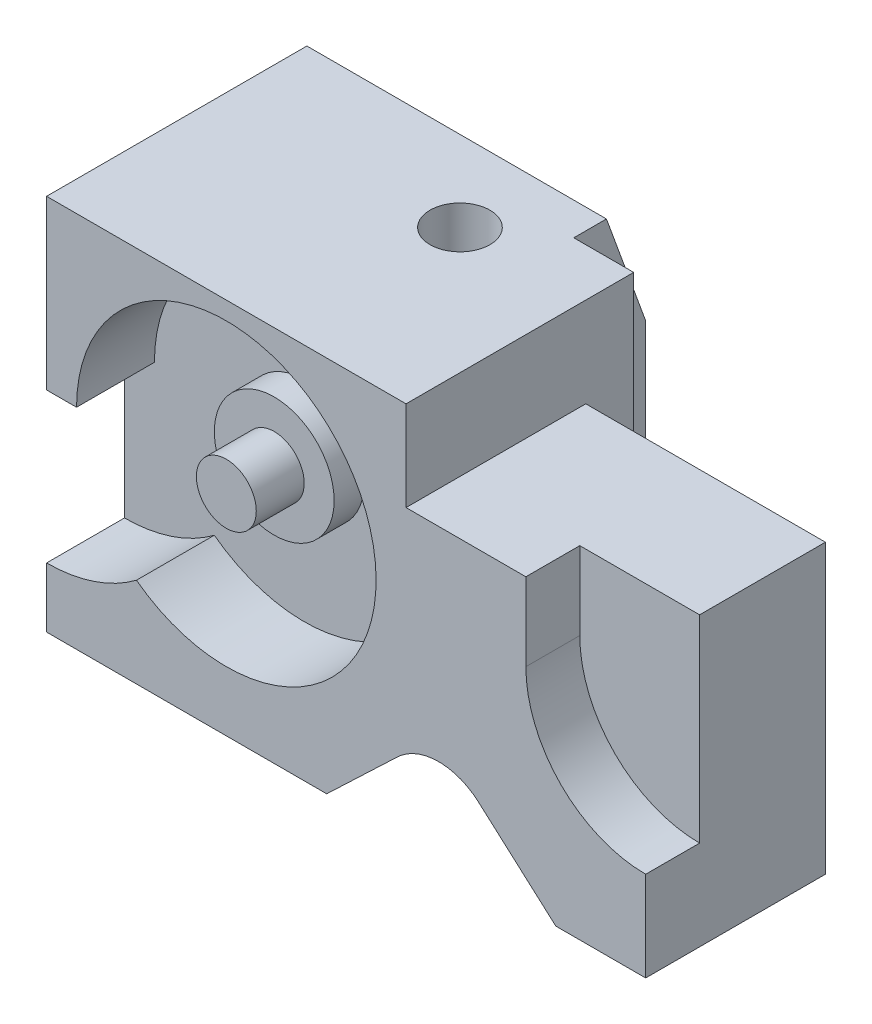
ISO-10303-21;
HEADER;
FILE_DESCRIPTION(('STEP AP214'),'2;1');
FILE_NAME('part.step','',(''),(''),'','','');
FILE_SCHEMA(('AUTOMOTIVE_DESIGN { 1 0 10303 214 1 1 1 1 }'));
ENDSEC;
DATA;
#1=APPLICATION_CONTEXT('core data for automotive mechanical design processes');
#2=APPLICATION_PROTOCOL_DEFINITION('international standard','automotive_design',2000,#1);
#3=PRODUCT_CONTEXT('',#1,'mechanical');
#4=PRODUCT('Part','Part','',(#3));
#5=PRODUCT_RELATED_PRODUCT_CATEGORY('part','',(#4));
#6=PRODUCT_DEFINITION_FORMATION('','',#4);
#7=PRODUCT_DEFINITION_CONTEXT('part definition',#1,'design');
#8=PRODUCT_DEFINITION('design','',#6,#7);
#9=PRODUCT_DEFINITION_SHAPE('','',#8);
#10=(LENGTH_UNIT() NAMED_UNIT(*) SI_UNIT(.MILLI.,.METRE.));
#11=(NAMED_UNIT(*) PLANE_ANGLE_UNIT() SI_UNIT($,.RADIAN.));
#12=(NAMED_UNIT(*) SI_UNIT($,.STERADIAN.) SOLID_ANGLE_UNIT());
#13=UNCERTAINTY_MEASURE_WITH_UNIT(LENGTH_MEASURE(1.E-05),#10,'distance_accuracy_value','');
#14=(GEOMETRIC_REPRESENTATION_CONTEXT(3) GLOBAL_UNCERTAINTY_ASSIGNED_CONTEXT((#13)) GLOBAL_UNIT_ASSIGNED_CONTEXT((#10,
#11,#12)) REPRESENTATION_CONTEXT('',''));
#15=CARTESIAN_POINT('',(0.,0.,0.));
#16=DIRECTION('',(0.,0.,1.));
#17=DIRECTION('',(1.,0.,0.));
#18=AXIS2_PLACEMENT_3D('',#15,#16,#17);
#19=CARTESIAN_POINT('',(-50.,63.,25.));
#20=DIRECTION('',(0.,0.,-1.));
#21=DIRECTION('',(-1.,0.,0.));
#22=AXIS2_PLACEMENT_3D('',#19,#20,#21);
#23=PLANE('',#22);
#24=DIRECTION('',(1.,0.,0.));
#25=VECTOR('',#24,1.);
#26=CARTESIAN_POINT('',(0.,35.,25.));
#27=LINE('',#26,#25);
#28=CARTESIAN_POINT('',(-50.,35.,25.));
#29=VERTEX_POINT('',#28);
#30=CARTESIAN_POINT('',(-45.,35.,25.));
#31=VERTEX_POINT('',#30);
#32=EDGE_CURVE('E266',#29,#31,#27,.T.);
#33=ORIENTED_EDGE('',*,*,#32,.T.);
#34=CARTESIAN_POINT('',(-20.,35.,25.));
#35=DIRECTION('',(0.,0.,1.));
#36=DIRECTION('',(1.,0.,0.));
#37=AXIS2_PLACEMENT_3D('',#34,#35,#36);
#38=CIRCLE('',#37,25.);
#39=CARTESIAN_POINT('',(-35.,15.,25.));
#40=VERTEX_POINT('',#39);
#41=EDGE_CURVE('E292',#40,#31,#38,.T.);
#42=ORIENTED_EDGE('',*,*,#41,.F.);
#43=CARTESIAN_POINT('',(-50.,35.,25.));
#44=DIRECTION('',(0.,0.,1.));
#45=DIRECTION('',(1.,0.,0.));
#46=AXIS2_PLACEMENT_3D('',#43,#44,#45);
#47=CIRCLE('',#46,25.);
#48=CARTESIAN_POINT('',(-50.,10.,25.));
#49=VERTEX_POINT('',#48);
#50=EDGE_CURVE('E264',#49,#40,#47,.T.);
#51=ORIENTED_EDGE('',*,*,#50,.F.);
#52=DIRECTION('',(0.,-1.,0.));
#53=VECTOR('',#52,1.);
#54=CARTESIAN_POINT('',(-50.,63.,25.));
#55=LINE('',#54,#53);
#56=CARTESIAN_POINT('',(-50.,0.,25.));
#57=VERTEX_POINT('',#56);
#58=EDGE_CURVE('E209',#49,#57,#55,.T.);
#59=ORIENTED_EDGE('',*,*,#58,.T.);
#60=DIRECTION('',(1.,0.,0.));
#61=VECTOR('',#60,1.);
#62=CARTESIAN_POINT('',(-50.,0.,25.));
#63=LINE('',#62,#61);
#64=CARTESIAN_POINT('',(-3.24667991345898,0.,25.));
#65=VERTEX_POINT('',#64);
#66=EDGE_CURVE('E351',#57,#65,#63,.T.);
#67=ORIENTED_EDGE('',*,*,#66,.T.);
#68=DIRECTION('',(0.724485251032931,0.689290302438494,0.));
#69=VECTOR('',#68,1.);
#70=CARTESIAN_POINT('',(-1.54256620012688,1.62132915083853,25.));
#71=LINE('',#70,#69);
#72=CARTESIAN_POINT('',(8.34365992738258,11.0272898487142,25.));
#73=VERTEX_POINT('',#72);
#74=EDGE_CURVE('E336',#65,#73,#71,.T.);
#75=ORIENTED_EDGE('',*,*,#74,.T.);
#76=CARTESIAN_POINT('',(15.4582363295416,4.,25.));
#77=DIRECTION('',(0.,0.,1.));
#78=DIRECTION('',(1.,0.,0.));
#79=AXIS2_PLACEMENT_3D('',#76,#77,#78);
#80=CIRCLE('',#79,9.99999999999999);
#81=CARTESIAN_POINT('',(22.1048169338786,11.4714768466516,25.));
#82=VERTEX_POINT('',#81);
#83=EDGE_CURVE('E335',#82,#73,#80,.T.);
#84=ORIENTED_EDGE('',*,*,#83,.F.);
#85=DIRECTION('',(0.747147684665161,-0.664658060433701,0.));
#86=VECTOR('',#85,1.);
#87=CARTESIAN_POINT('',(15.4619618054821,17.3809205831477,25.));
#88=LINE('',#87,#86);
#89=CARTESIAN_POINT('',(35.,0.,25.));
#90=VERTEX_POINT('',#89);
#91=EDGE_CURVE('E331',#82,#90,#88,.T.);
#92=ORIENTED_EDGE('',*,*,#91,.T.);
#93=CARTESIAN_POINT('',(50.,0.,25.));
#94=VERTEX_POINT('',#93);
#95=EDGE_CURVE('E359',#90,#94,#63,.T.);
#96=ORIENTED_EDGE('',*,*,#95,.T.);
#97=DIRECTION('',(0.,-1.,0.));
#98=VECTOR('',#97,1.);
#99=CARTESIAN_POINT('',(50.,63.,25.));
#100=LINE('',#99,#98);
#101=CARTESIAN_POINT('',(50.,15.,25.));
#102=VERTEX_POINT('',#101);
#103=EDGE_CURVE('E353',#102,#94,#100,.T.);
#104=ORIENTED_EDGE('',*,*,#103,.F.);
#105=CARTESIAN_POINT('',(50.,35.,25.));
#106=DIRECTION('',(0.,0.,1.));
#107=DIRECTION('',(1.,0.,0.));
#108=AXIS2_PLACEMENT_3D('',#105,#106,#107);
#109=CIRCLE('',#108,20.);
#110=CARTESIAN_POINT('',(30.,35.,25.));
#111=VERTEX_POINT('',#110);
#112=EDGE_CURVE('E319',#111,#102,#109,.T.);
#113=ORIENTED_EDGE('',*,*,#112,.F.);
#114=DIRECTION('',(0.,1.,0.));
#115=VECTOR('',#114,1.);
#116=CARTESIAN_POINT('',(30.,0.,25.));
#117=LINE('',#116,#115);
#118=CARTESIAN_POINT('',(30.,48.,25.));
#119=VERTEX_POINT('',#118);
#120=EDGE_CURVE('E312',#111,#119,#117,.T.);
#121=ORIENTED_EDGE('',*,*,#120,.T.);
#122=DIRECTION('',(1.,0.,0.));
#123=VECTOR('',#122,1.);
#124=CARTESIAN_POINT('',(50.,48.,25.));
#125=LINE('',#124,#123);
#126=CARTESIAN_POINT('',(10.,48.,25.));
#127=VERTEX_POINT('',#126);
#128=EDGE_CURVE('E304',#127,#119,#125,.T.);
#129=ORIENTED_EDGE('',*,*,#128,.F.);
#130=DIRECTION('',(0.,1.,0.));
#131=VECTOR('',#130,1.);
#132=CARTESIAN_POINT('',(10.,48.,25.));
#133=LINE('',#132,#131);
#134=CARTESIAN_POINT('',(10.,63.,25.));
#135=VERTEX_POINT('',#134);
#136=EDGE_CURVE('E310',#127,#135,#133,.T.);
#137=ORIENTED_EDGE('',*,*,#136,.T.);
#138=DIRECTION('',(1.,0.,0.));
#139=VECTOR('',#138,1.);
#140=CARTESIAN_POINT('',(-50.,63.,25.));
#141=LINE('',#140,#139);
#142=CARTESIAN_POINT('',(-50.,63.,25.));
#143=VERTEX_POINT('',#142);
#144=EDGE_CURVE('E348',#143,#135,#141,.T.);
#145=ORIENTED_EDGE('',*,*,#144,.F.);
#146=EDGE_CURVE('E203',#143,#29,#55,.T.);
#147=ORIENTED_EDGE('',*,*,#146,.T.);
#148=EDGE_LOOP('',(#33,#42,#51,#59,#67,#75,#84,#92,#96,#104,#113,#121,#129,#137,#145,#147));
#149=FACE_BOUND('',#148,.T.);
#150=ADVANCED_FACE('F39',(#149),#23,.F.);
#151=CARTESIAN_POINT('',(-50.,63.,-25.));
#152=DIRECTION('',(1.,0.,0.));
#153=DIRECTION('',(0.,0.,-1.));
#154=AXIS2_PLACEMENT_3D('',#151,#152,#153);
#155=PLANE('',#154);
#156=DIRECTION('',(0.,0.,1.));
#157=VECTOR('',#156,1.);
#158=CARTESIAN_POINT('',(-50.,63.,-25.));
#159=LINE('',#158,#157);
#160=CARTESIAN_POINT('',(-50.,63.,-18.4485357832084));
#161=VERTEX_POINT('',#160);
#162=EDGE_CURVE('E197',#161,#143,#159,.T.);
#163=ORIENTED_EDGE('',*,*,#162,.F.);
#164=DIRECTION('',(0.,0.93969262078591,0.342020143325666));
#165=VECTOR('',#164,1.);
#166=CARTESIAN_POINT('',(-50.,45.,-25.));
#167=LINE('',#166,#165);
#168=CARTESIAN_POINT('',(-50.,45.,-25.));
#169=VERTEX_POINT('',#168);
#170=EDGE_CURVE('E182',#169,#161,#167,.T.);
#171=ORIENTED_EDGE('',*,*,#170,.F.);
#172=DIRECTION('',(0.,-1.,0.));
#173=VECTOR('',#172,1.);
#174=CARTESIAN_POINT('',(-50.,63.,-25.));
#175=LINE('',#174,#173);
#176=CARTESIAN_POINT('',(-50.,0.,-25.));
#177=VERTEX_POINT('',#176);
#178=EDGE_CURVE('E195',#169,#177,#175,.T.);
#179=ORIENTED_EDGE('',*,*,#178,.T.);
#180=DIRECTION('',(0.,0.,1.));
#181=VECTOR('',#180,1.);
#182=CARTESIAN_POINT('',(-50.,0.,-25.));
#183=LINE('',#182,#181);
#184=EDGE_CURVE('E356',#177,#57,#183,.T.);
#185=ORIENTED_EDGE('',*,*,#184,.T.);
#186=ORIENTED_EDGE('',*,*,#58,.F.);
#187=DIRECTION('',(0.,0.,1.));
#188=VECTOR('',#187,1.);
#189=CARTESIAN_POINT('',(-50.,10.,12.));
#190=LINE('',#189,#188);
#191=CARTESIAN_POINT('',(-50.,10.,12.));
#192=VERTEX_POINT('',#191);
#193=EDGE_CURVE('E270',#192,#49,#190,.T.);
#194=ORIENTED_EDGE('',*,*,#193,.F.);
#195=DIRECTION('',(0.,-1.,0.));
#196=VECTOR('',#195,1.);
#197=CARTESIAN_POINT('',(-50.,0.,12.));
#198=LINE('',#197,#196);
#199=CARTESIAN_POINT('',(-50.,35.,12.));
#200=VERTEX_POINT('',#199);
#201=EDGE_CURVE('E261',#200,#192,#198,.T.);
#202=ORIENTED_EDGE('',*,*,#201,.F.);
#203=DIRECTION('',(0.,0.,1.));
#204=VECTOR('',#203,1.);
#205=CARTESIAN_POINT('',(-50.,35.,12.));
#206=LINE('',#205,#204);
#207=EDGE_CURVE('E274',#200,#29,#206,.T.);
#208=ORIENTED_EDGE('',*,*,#207,.T.);
#209=ORIENTED_EDGE('',*,*,#146,.F.);
#210=EDGE_LOOP('',(#163,#171,#179,#185,#186,#194,#202,#208,#209));
#211=FACE_BOUND('',#210,.T.);
#212=ADVANCED_FACE('F194',(#211),#155,.F.);
#213=CARTESIAN_POINT('',(-20.,35.,12.));
#214=DIRECTION('',(0.,0.,1.));
#215=DIRECTION('',(1.,0.,0.));
#216=AXIS2_PLACEMENT_3D('',#213,#214,#215);
#217=CYLINDRICAL_SURFACE('',#216,25.);
#218=DIRECTION('',(0.,0.,1.));
#219=VECTOR('',#218,1.);
#220=CARTESIAN_POINT('',(-45.,35.,12.));
#221=LINE('',#220,#219);
#222=CARTESIAN_POINT('',(-45.,35.,12.));
#223=VERTEX_POINT('',#222);
#224=EDGE_CURVE('E280',#223,#31,#221,.T.);
#225=ORIENTED_EDGE('',*,*,#224,.F.);
#226=CARTESIAN_POINT('',(-20.,35.,12.));
#227=DIRECTION('',(0.,0.,1.));
#228=DIRECTION('',(1.,0.,0.));
#229=AXIS2_PLACEMENT_3D('',#226,#227,#228);
#230=CIRCLE('',#229,25.);
#231=CARTESIAN_POINT('',(-35.,15.,12.));
#232=VERTEX_POINT('',#231);
#233=EDGE_CURVE('E294',#232,#223,#230,.T.);
#234=ORIENTED_EDGE('',*,*,#233,.F.);
#235=DIRECTION('',(0.,0.,1.));
#236=VECTOR('',#235,1.);
#237=CARTESIAN_POINT('',(-35.,15.,12.));
#238=LINE('',#237,#236);
#239=EDGE_CURVE('E277',#232,#40,#238,.T.);
#240=ORIENTED_EDGE('',*,*,#239,.T.);
#241=ORIENTED_EDGE('',*,*,#41,.T.);
#242=EDGE_LOOP('',(#225,#234,#240,#241));
#243=FACE_BOUND('',#242,.T.);
#244=ADVANCED_FACE('F432',(#243),#217,.F.);
#245=CARTESIAN_POINT('',(0.,63.,0.));
#246=DIRECTION('',(0.,1.,0.));
#247=DIRECTION('',(0.,0.,1.));
#248=AXIS2_PLACEMENT_3D('',#245,#246,#247);
#249=PLANE('',#248);
#250=DIRECTION('',(-1.,0.,0.));
#251=VECTOR('',#250,1.);
#252=CARTESIAN_POINT('',(67.,63.,-18.4485357832084));
#253=LINE('',#252,#251);
#254=CARTESIAN_POINT('',(0.,63.,-18.4485357832084));
#255=VERTEX_POINT('',#254);
#256=EDGE_CURVE('E53',#255,#161,#253,.T.);
#257=ORIENTED_EDGE('',*,*,#256,.T.);
#258=ORIENTED_EDGE('',*,*,#162,.T.);
#259=ORIENTED_EDGE('',*,*,#144,.T.);
#260=DIRECTION('',(0.,0.,1.));
#261=VECTOR('',#260,1.);
#262=CARTESIAN_POINT('',(10.,63.,25.));
#263=LINE('',#262,#261);
#264=CARTESIAN_POINT('',(10.,63.,-13.));
#265=VERTEX_POINT('',#264);
#266=EDGE_CURVE('E300',#265,#135,#263,.T.);
#267=ORIENTED_EDGE('',*,*,#266,.F.);
#268=DIRECTION('',(1.,0.,0.));
#269=VECTOR('',#268,1.);
#270=CARTESIAN_POINT('',(10.,63.,-13.));
#271=LINE('',#270,#269);
#272=CARTESIAN_POINT('',(0.,63.,-13.));
#273=VERTEX_POINT('',#272);
#274=EDGE_CURVE('E247',#273,#265,#271,.T.);
#275=ORIENTED_EDGE('',*,*,#274,.F.);
#276=DIRECTION('',(0.,0.,1.));
#277=VECTOR('',#276,1.);
#278=CARTESIAN_POINT('',(0.,63.,-13.));
#279=LINE('',#278,#277);
#280=EDGE_CURVE('E246',#255,#273,#279,.T.);
#281=ORIENTED_EDGE('',*,*,#280,.F.);
#282=EDGE_LOOP('',(#257,#258,#259,#267,#275,#281));
#283=FACE_BOUND('',#282,.T.);
#284=CARTESIAN_POINT('',(-11.,63.,-4.99999999999998));
#285=DIRECTION('',(0.,1.,0.));
#286=DIRECTION('',(0.,0.,1.));
#287=AXIS2_PLACEMENT_3D('',#284,#285,#286);
#288=CIRCLE('',#287,5.);
#289=CARTESIAN_POINT('',(-11.,63.,0.));
#290=VERTEX_POINT('',#289);
#291=EDGE_CURVE('E218',#290,#290,#288,.T.);
#292=ORIENTED_EDGE('',*,*,#291,.F.);
#293=EDGE_LOOP('',(#292));
#294=FACE_BOUND('',#293,.T.);
#295=ADVANCED_FACE('F425',(#283,#294),#249,.T.);
#296=CARTESIAN_POINT('',(50.,63.,-25.));
#297=DIRECTION('',(0.,0.,1.));
#298=DIRECTION('',(1.,0.,0.));
#299=AXIS2_PLACEMENT_3D('',#296,#297,#298);
#300=PLANE('',#299);
#301=ORIENTED_EDGE('',*,*,#178,.F.);
#302=DIRECTION('',(-1.,0.,0.));
#303=VECTOR('',#302,1.);
#304=CARTESIAN_POINT('',(67.,45.,-25.));
#305=LINE('',#304,#303);
#306=CARTESIAN_POINT('',(0.,45.,-25.));
#307=VERTEX_POINT('',#306);
#308=EDGE_CURVE('E179',#307,#169,#305,.T.);
#309=ORIENTED_EDGE('',*,*,#308,.F.);
#310=DIRECTION('',(0.,1.,0.));
#311=VECTOR('',#310,1.);
#312=CARTESIAN_POINT('',(0.,-54.,-25.));
#313=LINE('',#312,#311);
#314=CARTESIAN_POINT('',(0.,3.08895864516005,-25.));
#315=VERTEX_POINT('',#314);
#316=EDGE_CURVE('E252',#315,#307,#313,.T.);
#317=ORIENTED_EDGE('',*,*,#316,.F.);
#318=DIRECTION('',(0.724485251032931,0.689290302438494,0.));
#319=VECTOR('',#318,1.);
#320=CARTESIAN_POINT('',(56.1623591892788,56.5229926659267,-25.));
#321=LINE('',#320,#319);
#322=CARTESIAN_POINT('',(-3.24667991345898,0.,-25.));
#323=VERTEX_POINT('',#322);
#324=EDGE_CURVE('E343',#323,#315,#321,.T.);
#325=ORIENTED_EDGE('',*,*,#324,.F.);
#326=DIRECTION('',(-1.,0.,0.));
#327=VECTOR('',#326,1.);
#328=CARTESIAN_POINT('',(50.,0.,-25.));
#329=LINE('',#328,#327);
#330=EDGE_CURVE('E201',#323,#177,#329,.T.);
#331=ORIENTED_EDGE('',*,*,#330,.T.);
#332=EDGE_LOOP('',(#301,#309,#317,#325,#331));
#333=FACE_BOUND('',#332,.T.);
#334=ADVANCED_FACE('F199',(#333),#300,.F.);
#335=CARTESIAN_POINT('',(0.,0.,0.));
#336=DIRECTION('',(0.,1.,0.));
#337=DIRECTION('',(0.,0.,1.));
#338=AXIS2_PLACEMENT_3D('',#335,#336,#337);
#339=PLANE('',#338);
#340=DIRECTION('',(0.,0.,1.));
#341=VECTOR('',#340,1.);
#342=CARTESIAN_POINT('',(35.,0.,0.));
#343=LINE('',#342,#341);
#344=CARTESIAN_POINT('',(35.,0.,-4.99999999999998));
#345=VERTEX_POINT('',#344);
#346=EDGE_CURVE('E207',#345,#90,#343,.T.);
#347=ORIENTED_EDGE('',*,*,#346,.F.);
#348=DIRECTION('',(1.,0.,0.));
#349=VECTOR('',#348,1.);
#350=CARTESIAN_POINT('',(0.,0.,-4.99999999999998));
#351=LINE('',#350,#349);
#352=CARTESIAN_POINT('',(50.,0.,-4.99999999999998));
#353=VERTEX_POINT('',#352);
#354=EDGE_CURVE('E243',#345,#353,#351,.T.);
#355=ORIENTED_EDGE('',*,*,#354,.T.);
#356=DIRECTION('',(0.,0.,-1.));
#357=VECTOR('',#356,1.);
#358=CARTESIAN_POINT('',(50.,0.,0.));
#359=LINE('',#358,#357);
#360=EDGE_CURVE('E349',#94,#353,#359,.T.);
#361=ORIENTED_EDGE('',*,*,#360,.F.);
#362=ORIENTED_EDGE('',*,*,#95,.F.);
#363=EDGE_LOOP('',(#347,#355,#361,#362));
#364=FACE_BOUND('',#363,.T.);
#365=ADVANCED_FACE('F391',(#364),#339,.F.);
#366=CARTESIAN_POINT('',(-11.,0.,-4.99999999999998));
#367=DIRECTION('',(0.,1.,0.));
#368=DIRECTION('',(0.,0.,1.));
#369=AXIS2_PLACEMENT_3D('',#366,#367,#368);
#370=CIRCLE('',#369,5.);
#371=CARTESIAN_POINT('',(-11.,0.,0.));
#372=VERTEX_POINT('',#371);
#373=EDGE_CURVE('E220',#372,#372,#370,.T.);
#374=ORIENTED_EDGE('',*,*,#373,.T.);
#375=EDGE_LOOP('',(#374));
#376=FACE_BOUND('',#375,.T.);
#377=DIRECTION('',(0.,0.,-1.));
#378=VECTOR('',#377,1.);
#379=CARTESIAN_POINT('',(-3.24667991345897,0.,0.));
#380=LINE('',#379,#378);
#381=EDGE_CURVE('E204',#65,#323,#380,.T.);
#382=ORIENTED_EDGE('',*,*,#381,.F.);
#383=ORIENTED_EDGE('',*,*,#66,.F.);
#384=ORIENTED_EDGE('',*,*,#184,.F.);
#385=ORIENTED_EDGE('',*,*,#330,.F.);
#386=EDGE_LOOP('',(#382,#383,#384,#385));
#387=FACE_BOUND('',#386,.T.);
#388=ADVANCED_FACE('F373',(#376,#387),#339,.F.);
#389=CARTESIAN_POINT('',(50.,63.,0.));
#390=DIRECTION('',(-1.,0.,0.));
#391=DIRECTION('',(0.,0.,1.));
#392=AXIS2_PLACEMENT_3D('',#389,#390,#391);
#393=PLANE('',#392);
#394=ORIENTED_EDGE('',*,*,#360,.T.);
#395=DIRECTION('',(0.,1.,0.));
#396=VECTOR('',#395,1.);
#397=CARTESIAN_POINT('',(50.,-69.,-4.99999999999998));
#398=LINE('',#397,#396);
#399=CARTESIAN_POINT('',(50.,48.,-4.99999999999998));
#400=VERTEX_POINT('',#399);
#401=EDGE_CURVE('E224',#353,#400,#398,.T.);
#402=ORIENTED_EDGE('',*,*,#401,.T.);
#403=DIRECTION('',(0.,0.,-1.));
#404=VECTOR('',#403,1.);
#405=CARTESIAN_POINT('',(50.,48.,-25.));
#406=LINE('',#405,#404);
#407=CARTESIAN_POINT('',(50.,48.,16.));
#408=VERTEX_POINT('',#407);
#409=EDGE_CURVE('E297',#408,#400,#406,.T.);
#410=ORIENTED_EDGE('',*,*,#409,.F.);
#411=DIRECTION('',(0.,1.,0.));
#412=VECTOR('',#411,1.);
#413=CARTESIAN_POINT('',(50.,0.,16.));
#414=LINE('',#413,#412);
#415=CARTESIAN_POINT('',(50.,15.,16.));
#416=VERTEX_POINT('',#415);
#417=EDGE_CURVE('E324',#416,#408,#414,.T.);
#418=ORIENTED_EDGE('',*,*,#417,.F.);
#419=DIRECTION('',(0.,0.,1.));
#420=VECTOR('',#419,1.);
#421=CARTESIAN_POINT('',(50.,15.,16.));
#422=LINE('',#421,#420);
#423=EDGE_CURVE('E329',#416,#102,#422,.T.);
#424=ORIENTED_EDGE('',*,*,#423,.T.);
#425=ORIENTED_EDGE('',*,*,#103,.T.);
#426=EDGE_LOOP('',(#394,#402,#410,#418,#424,#425));
#427=FACE_BOUND('',#426,.T.);
#428=ADVANCED_FACE('F41',(#427),#393,.F.);
#429=CARTESIAN_POINT('',(15.4582363295416,4.,-38.));
#430=DIRECTION('',(0.,0.,1.));
#431=DIRECTION('',(1.,0.,0.));
#432=AXIS2_PLACEMENT_3D('',#429,#430,#431);
#433=CYLINDRICAL_SURFACE('',#432,9.99999999999999);
#434=CARTESIAN_POINT('',(15.4582363295416,4.,-13.));
#435=DIRECTION('',(0.,0.,1.));
#436=DIRECTION('',(1.,0.,0.));
#437=AXIS2_PLACEMENT_3D('',#434,#435,#436);
#438=CIRCLE('',#437,9.99999999999999);
#439=CARTESIAN_POINT('',(8.34365992738258,11.0272898487142,-13.));
#440=VERTEX_POINT('',#439);
#441=CARTESIAN_POINT('',(10.,12.3790009052913,-13.));
#442=VERTEX_POINT('',#441);
#443=EDGE_CURVE('E257',#440,#442,#438,.F.);
#444=ORIENTED_EDGE('',*,*,#443,.T.);
#445=DIRECTION('',(0.,0.,1.));
#446=VECTOR('',#445,1.);
#447=CARTESIAN_POINT('',(10.,12.3790009052913,-38.));
#448=LINE('',#447,#446);
#449=CARTESIAN_POINT('',(10.,12.3790009052913,-4.99999999999998));
#450=VERTEX_POINT('',#449);
#451=EDGE_CURVE('E231',#442,#450,#448,.T.);
#452=ORIENTED_EDGE('',*,*,#451,.T.);
#453=CARTESIAN_POINT('',(15.4582363295416,4.,-4.99999999999998));
#454=DIRECTION('',(0.,0.,1.));
#455=DIRECTION('',(1.,0.,0.));
#456=AXIS2_PLACEMENT_3D('',#453,#454,#455);
#457=CIRCLE('',#456,9.99999999999999);
#458=CARTESIAN_POINT('',(22.1048169338786,11.4714768466516,-4.99999999999998));
#459=VERTEX_POINT('',#458);
#460=EDGE_CURVE('E239',#450,#459,#457,.F.);
#461=ORIENTED_EDGE('',*,*,#460,.T.);
#462=DIRECTION('',(0.,0.,1.));
#463=VECTOR('',#462,1.);
#464=CARTESIAN_POINT('',(22.1048169338786,11.4714768466516,-38.));
#465=LINE('',#464,#463);
#466=EDGE_CURVE('E344',#459,#82,#465,.T.);
#467=ORIENTED_EDGE('',*,*,#466,.T.);
#468=ORIENTED_EDGE('',*,*,#83,.T.);
#469=DIRECTION('',(0.,0.,1.));
#470=VECTOR('',#469,1.);
#471=CARTESIAN_POINT('',(8.34365992738258,11.0272898487142,-38.));
#472=LINE('',#471,#470);
#473=EDGE_CURVE('E341',#440,#73,#472,.T.);
#474=ORIENTED_EDGE('',*,*,#473,.F.);
#475=EDGE_LOOP('',(#444,#452,#461,#467,#468,#474));
#476=FACE_BOUND('',#475,.T.);
#477=ADVANCED_FACE('F383',(#476),#433,.F.);
#478=CARTESIAN_POINT('',(15.4619618054821,17.3809205831477,-38.));
#479=DIRECTION('',(-0.664658060433701,-0.747147684665161,0.));
#480=DIRECTION('',(0.747147684665161,-0.664658060433701,0.));
#481=AXIS2_PLACEMENT_3D('',#478,#479,#480);
#482=PLANE('',#481);
#483=DIRECTION('',(-0.747147684665161,0.664658060433701,0.));
#484=VECTOR('',#483,1.);
#485=CARTESIAN_POINT('',(15.4619618054821,17.3809205831477,-4.99999999999998));
#486=LINE('',#485,#484);
#487=EDGE_CURVE('E238',#345,#459,#486,.T.);
#488=ORIENTED_EDGE('',*,*,#487,.F.);
#489=ORIENTED_EDGE('',*,*,#346,.T.);
#490=ORIENTED_EDGE('',*,*,#91,.F.);
#491=ORIENTED_EDGE('',*,*,#466,.F.);
#492=EDGE_LOOP('',(#488,#489,#490,#491));
#493=FACE_BOUND('',#492,.T.);
#494=ADVANCED_FACE('F469',(#493),#482,.T.);
#495=CARTESIAN_POINT('',(-1.54256620012688,1.62132915083853,-38.));
#496=DIRECTION('',(0.689290302438494,-0.724485251032931,0.));
#497=DIRECTION('',(0.724485251032931,0.689290302438494,0.));
#498=AXIS2_PLACEMENT_3D('',#495,#496,#497);
#499=PLANE('',#498);
#500=DIRECTION('',(-0.724485251032931,-0.689290302438494,0.));
#501=VECTOR('',#500,1.);
#502=CARTESIAN_POINT('',(-1.54256620012688,1.62132915083853,-13.));
#503=LINE('',#502,#501);
#504=CARTESIAN_POINT('',(0.,3.08895864516005,-13.));
#505=VERTEX_POINT('',#504);
#506=EDGE_CURVE('E251',#440,#505,#503,.T.);
#507=ORIENTED_EDGE('',*,*,#506,.F.);
#508=ORIENTED_EDGE('',*,*,#473,.T.);
#509=ORIENTED_EDGE('',*,*,#74,.F.);
#510=ORIENTED_EDGE('',*,*,#381,.T.);
#511=ORIENTED_EDGE('',*,*,#324,.T.);
#512=DIRECTION('',(0.,0.,-1.));
#513=VECTOR('',#512,1.);
#514=CARTESIAN_POINT('',(0.,3.08895864516005,-38.));
#515=LINE('',#514,#513);
#516=EDGE_CURVE('E50',#505,#315,#515,.T.);
#517=ORIENTED_EDGE('',*,*,#516,.F.);
#518=EDGE_LOOP('',(#507,#508,#509,#510,#511,#517));
#519=FACE_BOUND('',#518,.T.);
#520=ADVANCED_FACE('F376',(#519),#499,.T.);
#521=CARTESIAN_POINT('',(30.,0.,16.));
#522=DIRECTION('',(1.,0.,0.));
#523=DIRECTION('',(0.,0.,-1.));
#524=AXIS2_PLACEMENT_3D('',#521,#522,#523);
#525=PLANE('',#524);
#526=DIRECTION('',(0.,0.,-1.));
#527=VECTOR('',#526,1.);
#528=CARTESIAN_POINT('',(30.,48.,16.));
#529=LINE('',#528,#527);
#530=CARTESIAN_POINT('',(30.,48.,16.));
#531=VERTEX_POINT('',#530);
#532=EDGE_CURVE('E311',#119,#531,#529,.T.);
#533=ORIENTED_EDGE('',*,*,#532,.F.);
#534=ORIENTED_EDGE('',*,*,#120,.F.);
#535=DIRECTION('',(0.,0.,1.));
#536=VECTOR('',#535,1.);
#537=CARTESIAN_POINT('',(30.,35.,16.));
#538=LINE('',#537,#536);
#539=CARTESIAN_POINT('',(30.,35.,16.));
#540=VERTEX_POINT('',#539);
#541=EDGE_CURVE('E323',#540,#111,#538,.T.);
#542=ORIENTED_EDGE('',*,*,#541,.F.);
#543=DIRECTION('',(0.,1.,0.));
#544=VECTOR('',#543,1.);
#545=CARTESIAN_POINT('',(30.,0.,16.));
#546=LINE('',#545,#544);
#547=EDGE_CURVE('E313',#540,#531,#546,.T.);
#548=ORIENTED_EDGE('',*,*,#547,.T.);
#549=EDGE_LOOP('',(#533,#534,#542,#548));
#550=FACE_BOUND('',#549,.T.);
#551=ADVANCED_FACE('F408',(#550),#525,.T.);
#552=CARTESIAN_POINT('',(50.,35.,16.));
#553=DIRECTION('',(0.,0.,1.));
#554=DIRECTION('',(1.,0.,0.));
#555=AXIS2_PLACEMENT_3D('',#552,#553,#554);
#556=CYLINDRICAL_SURFACE('',#555,20.);
#557=ORIENTED_EDGE('',*,*,#112,.T.);
#558=ORIENTED_EDGE('',*,*,#423,.F.);
#559=CARTESIAN_POINT('',(50.,35.,16.));
#560=DIRECTION('',(0.,0.,1.));
#561=DIRECTION('',(1.,0.,0.));
#562=AXIS2_PLACEMENT_3D('',#559,#560,#561);
#563=CIRCLE('',#562,20.);
#564=EDGE_CURVE('E320',#540,#416,#563,.T.);
#565=ORIENTED_EDGE('',*,*,#564,.F.);
#566=ORIENTED_EDGE('',*,*,#541,.T.);
#567=EDGE_LOOP('',(#557,#558,#565,#566));
#568=FACE_BOUND('',#567,.T.);
#569=ADVANCED_FACE('F414',(#568),#556,.F.);
#570=CARTESIAN_POINT('',(0.,0.,16.));
#571=DIRECTION('',(0.,0.,1.));
#572=DIRECTION('',(1.,0.,0.));
#573=AXIS2_PLACEMENT_3D('',#570,#571,#572);
#574=PLANE('',#573);
#575=DIRECTION('',(1.,0.,0.));
#576=VECTOR('',#575,1.);
#577=CARTESIAN_POINT('',(0.,48.,16.));
#578=LINE('',#577,#576);
#579=EDGE_CURVE('E213',#531,#408,#578,.T.);
#580=ORIENTED_EDGE('',*,*,#579,.F.);
#581=ORIENTED_EDGE('',*,*,#547,.F.);
#582=ORIENTED_EDGE('',*,*,#564,.T.);
#583=ORIENTED_EDGE('',*,*,#417,.T.);
#584=EDGE_LOOP('',(#580,#581,#582,#583));
#585=FACE_BOUND('',#584,.T.);
#586=ADVANCED_FACE('F409',(#585),#574,.T.);
#587=CARTESIAN_POINT('',(10.,48.,25.));
#588=DIRECTION('',(-1.,0.,0.));
#589=DIRECTION('',(0.,0.,1.));
#590=AXIS2_PLACEMENT_3D('',#587,#588,#589);
#591=PLANE('',#590);
#592=DIRECTION('',(0.,0.,1.));
#593=VECTOR('',#592,1.);
#594=CARTESIAN_POINT('',(10.,48.,25.));
#595=LINE('',#594,#593);
#596=CARTESIAN_POINT('',(10.,48.,-4.99999999999998));
#597=VERTEX_POINT('',#596);
#598=EDGE_CURVE('E303',#597,#127,#595,.T.);
#599=ORIENTED_EDGE('',*,*,#598,.F.);
#600=DIRECTION('',(0.,1.,0.));
#601=VECTOR('',#600,1.);
#602=CARTESIAN_POINT('',(10.,-69.,-4.99999999999998));
#603=LINE('',#602,#601);
#604=EDGE_CURVE('E233',#450,#597,#603,.T.);
#605=ORIENTED_EDGE('',*,*,#604,.F.);
#606=ORIENTED_EDGE('',*,*,#451,.F.);
#607=DIRECTION('',(0.,1.,0.));
#608=VECTOR('',#607,1.);
#609=CARTESIAN_POINT('',(10.,-54.,-13.));
#610=LINE('',#609,#608);
#611=EDGE_CURVE('E255',#442,#265,#610,.T.);
#612=ORIENTED_EDGE('',*,*,#611,.T.);
#613=ORIENTED_EDGE('',*,*,#266,.T.);
#614=ORIENTED_EDGE('',*,*,#136,.F.);
#615=EDGE_LOOP('',(#599,#605,#606,#612,#613,#614));
#616=FACE_BOUND('',#615,.T.);
#617=ADVANCED_FACE('F418',(#616),#591,.F.);
#618=CARTESIAN_POINT('',(0.,48.,0.));
#619=DIRECTION('',(0.,-1.,0.));
#620=DIRECTION('',(0.,0.,-1.));
#621=AXIS2_PLACEMENT_3D('',#618,#619,#620);
#622=PLANE('',#621);
#623=ORIENTED_EDGE('',*,*,#409,.T.);
#624=DIRECTION('',(1.,0.,0.));
#625=VECTOR('',#624,1.);
#626=CARTESIAN_POINT('',(20.,48.,-4.99999999999998));
#627=LINE('',#626,#625);
#628=EDGE_CURVE('E216',#597,#400,#627,.T.);
#629=ORIENTED_EDGE('',*,*,#628,.F.);
#630=ORIENTED_EDGE('',*,*,#598,.T.);
#631=ORIENTED_EDGE('',*,*,#128,.T.);
#632=ORIENTED_EDGE('',*,*,#532,.T.);
#633=ORIENTED_EDGE('',*,*,#579,.T.);
#634=EDGE_LOOP('',(#623,#629,#630,#631,#632,#633));
#635=FACE_BOUND('',#634,.T.);
#636=ADVANCED_FACE('F400',(#635),#622,.F.);
#637=CARTESIAN_POINT('',(-20.,35.,12.));
#638=DIRECTION('',(0.,0.,1.));
#639=DIRECTION('',(1.,0.,0.));
#640=AXIS2_PLACEMENT_3D('',#637,#638,#639);
#641=PLANE('',#640);
#642=CARTESIAN_POINT('',(-20.,35.,12.));
#643=DIRECTION('',(0.,0.,1.));
#644=DIRECTION('',(1.,0.,0.));
#645=AXIS2_PLACEMENT_3D('',#642,#643,#644);
#646=CIRCLE('',#645,10.);
#647=CARTESIAN_POINT('',(-9.99999999999999,35.,12.));
#648=VERTEX_POINT('',#647);
#649=EDGE_CURVE('E286',#648,#648,#646,.T.);
#650=ORIENTED_EDGE('',*,*,#649,.F.);
#651=EDGE_LOOP('',(#650));
#652=FACE_BOUND('',#651,.T.);
#653=ORIENTED_EDGE('',*,*,#233,.T.);
#654=DIRECTION('',(1.,0.,0.));
#655=VECTOR('',#654,1.);
#656=CARTESIAN_POINT('',(0.,35.,12.));
#657=LINE('',#656,#655);
#658=EDGE_CURVE('E269',#200,#223,#657,.T.);
#659=ORIENTED_EDGE('',*,*,#658,.F.);
#660=ORIENTED_EDGE('',*,*,#201,.T.);
#661=CARTESIAN_POINT('',(-50.,35.,12.));
#662=DIRECTION('',(0.,0.,1.));
#663=DIRECTION('',(1.,0.,0.));
#664=AXIS2_PLACEMENT_3D('',#661,#662,#663);
#665=CIRCLE('',#664,25.);
#666=EDGE_CURVE('E64',#192,#232,#665,.T.);
#667=ORIENTED_EDGE('',*,*,#666,.T.);
#668=EDGE_LOOP('',(#653,#659,#660,#667));
#669=FACE_BOUND('',#668,.T.);
#670=ADVANCED_FACE('F431',(#652,#669),#641,.T.);
#671=CARTESIAN_POINT('',(-20.,35.,17.));
#672=DIRECTION('',(0.,0.,-1.));
#673=DIRECTION('',(-1.,0.,0.));
#674=AXIS2_PLACEMENT_3D('',#671,#672,#673);
#675=CYLINDRICAL_SURFACE('',#674,10.);
#676=CARTESIAN_POINT('',(-20.,35.,17.));
#677=DIRECTION('',(0.,0.,1.));
#678=DIRECTION('',(1.,0.,0.));
#679=AXIS2_PLACEMENT_3D('',#676,#677,#678);
#680=CIRCLE('',#679,10.);
#681=CARTESIAN_POINT('',(-9.99999999999999,35.,17.));
#682=VERTEX_POINT('',#681);
#683=EDGE_CURVE('E288',#682,#682,#680,.T.);
#684=ORIENTED_EDGE('',*,*,#683,.F.);
#685=EDGE_LOOP('',(#684));
#686=FACE_BOUND('',#685,.T.);
#687=ORIENTED_EDGE('',*,*,#649,.T.);
#688=EDGE_LOOP('',(#687));
#689=FACE_BOUND('',#688,.T.);
#690=ADVANCED_FACE('F487',(#686,#689),#675,.T.);
#691=CARTESIAN_POINT('',(-20.,35.,17.));
#692=DIRECTION('',(0.,0.,1.));
#693=DIRECTION('',(1.,0.,0.));
#694=AXIS2_PLACEMENT_3D('',#691,#692,#693);
#695=PLANE('',#694);
#696=CARTESIAN_POINT('',(-20.,35.,17.));
#697=DIRECTION('',(0.,0.,1.));
#698=DIRECTION('',(1.,0.,0.));
#699=AXIS2_PLACEMENT_3D('',#696,#697,#698);
#700=CIRCLE('',#699,5.);
#701=CARTESIAN_POINT('',(-15.,35.,17.));
#702=VERTEX_POINT('',#701);
#703=EDGE_CURVE('E217',#702,#702,#700,.T.);
#704=ORIENTED_EDGE('',*,*,#703,.F.);
#705=EDGE_LOOP('',(#704));
#706=FACE_BOUND('',#705,.T.);
#707=ORIENTED_EDGE('',*,*,#683,.T.);
#708=EDGE_LOOP('',(#707));
#709=FACE_BOUND('',#708,.T.);
#710=ADVANCED_FACE('F493',(#706,#709),#695,.T.);
#711=CARTESIAN_POINT('',(-20.,35.,25.));
#712=DIRECTION('',(0.,0.,-1.));
#713=DIRECTION('',(-1.,0.,0.));
#714=AXIS2_PLACEMENT_3D('',#711,#712,#713);
#715=CYLINDRICAL_SURFACE('',#714,5.);
#716=CARTESIAN_POINT('',(-20.,35.,25.));
#717=DIRECTION('',(0.,0.,1.));
#718=DIRECTION('',(1.,0.,0.));
#719=AXIS2_PLACEMENT_3D('',#716,#717,#718);
#720=CIRCLE('',#719,5.);
#721=CARTESIAN_POINT('',(-15.,35.,25.));
#722=VERTEX_POINT('',#721);
#723=EDGE_CURVE('E276',#722,#722,#720,.T.);
#724=ORIENTED_EDGE('',*,*,#723,.F.);
#725=EDGE_LOOP('',(#724));
#726=FACE_BOUND('',#725,.T.);
#727=ORIENTED_EDGE('',*,*,#703,.T.);
#728=EDGE_LOOP('',(#727));
#729=FACE_BOUND('',#728,.T.);
#730=ADVANCED_FACE('F492',(#726,#729),#715,.T.);
#731=CARTESIAN_POINT('',(-20.,35.,25.));
#732=DIRECTION('',(0.,0.,1.));
#733=DIRECTION('',(1.,0.,0.));
#734=AXIS2_PLACEMENT_3D('',#731,#732,#733);
#735=PLANE('',#734);
#736=ORIENTED_EDGE('',*,*,#723,.T.);
#737=EDGE_LOOP('',(#736));
#738=FACE_BOUND('',#737,.T.);
#739=ADVANCED_FACE('F447',(#738),#735,.T.);
#740=CARTESIAN_POINT('',(0.,35.,12.));
#741=DIRECTION('',(0.,-1.,0.));
#742=DIRECTION('',(0.,0.,-1.));
#743=AXIS2_PLACEMENT_3D('',#740,#741,#742);
#744=PLANE('',#743);
#745=ORIENTED_EDGE('',*,*,#32,.F.);
#746=ORIENTED_EDGE('',*,*,#207,.F.);
#747=ORIENTED_EDGE('',*,*,#658,.T.);
#748=ORIENTED_EDGE('',*,*,#224,.T.);
#749=EDGE_LOOP('',(#745,#746,#747,#748));
#750=FACE_BOUND('',#749,.T.);
#751=ADVANCED_FACE('F429',(#750),#744,.T.);
#752=CARTESIAN_POINT('',(-50.,35.,12.));
#753=DIRECTION('',(0.,0.,1.));
#754=DIRECTION('',(1.,0.,0.));
#755=AXIS2_PLACEMENT_3D('',#752,#753,#754);
#756=CYLINDRICAL_SURFACE('',#755,25.);
#757=ORIENTED_EDGE('',*,*,#50,.T.);
#758=ORIENTED_EDGE('',*,*,#239,.F.);
#759=ORIENTED_EDGE('',*,*,#666,.F.);
#760=ORIENTED_EDGE('',*,*,#193,.T.);
#761=EDGE_LOOP('',(#757,#758,#759,#760));
#762=FACE_BOUND('',#761,.T.);
#763=ADVANCED_FACE('F436',(#762),#756,.F.);
#764=CARTESIAN_POINT('',(10.,-54.,-13.));
#765=DIRECTION('',(0.,0.,1.));
#766=DIRECTION('',(1.,0.,0.));
#767=AXIS2_PLACEMENT_3D('',#764,#765,#766);
#768=PLANE('',#767);
#769=ORIENTED_EDGE('',*,*,#506,.T.);
#770=DIRECTION('',(0.,1.,0.));
#771=VECTOR('',#770,1.);
#772=CARTESIAN_POINT('',(0.,-54.,-13.));
#773=LINE('',#772,#771);
#774=EDGE_CURVE('E253',#505,#273,#773,.T.);
#775=ORIENTED_EDGE('',*,*,#774,.T.);
#776=ORIENTED_EDGE('',*,*,#274,.T.);
#777=ORIENTED_EDGE('',*,*,#611,.F.);
#778=ORIENTED_EDGE('',*,*,#443,.F.);
#779=EDGE_LOOP('',(#769,#775,#776,#777,#778));
#780=FACE_BOUND('',#779,.T.);
#781=ADVANCED_FACE('F438',(#780),#768,.F.);
#782=CARTESIAN_POINT('',(0.,-54.,-13.));
#783=DIRECTION('',(-1.,0.,0.));
#784=DIRECTION('',(0.,0.,1.));
#785=AXIS2_PLACEMENT_3D('',#782,#783,#784);
#786=PLANE('',#785);
#787=ORIENTED_EDGE('',*,*,#316,.T.);
#788=DIRECTION('',(0.,0.93969262078591,0.342020143325666));
#789=VECTOR('',#788,1.);
#790=CARTESIAN_POINT('',(0.,-38.5624742762705,-55.4142533381973));
#791=LINE('',#790,#789);
#792=EDGE_CURVE('E11',#307,#255,#791,.T.);
#793=ORIENTED_EDGE('',*,*,#792,.T.);
#794=ORIENTED_EDGE('',*,*,#280,.T.);
#795=ORIENTED_EDGE('',*,*,#774,.F.);
#796=ORIENTED_EDGE('',*,*,#516,.T.);
#797=EDGE_LOOP('',(#787,#793,#794,#795,#796));
#798=FACE_BOUND('',#797,.T.);
#799=ADVANCED_FACE('F378',(#798),#786,.F.);
#800=CARTESIAN_POINT('',(20.,-69.,-4.99999999999998));
#801=DIRECTION('',(0.,0.,1.));
#802=DIRECTION('',(1.,0.,0.));
#803=AXIS2_PLACEMENT_3D('',#800,#801,#802);
#804=PLANE('',#803);
#805=ORIENTED_EDGE('',*,*,#487,.T.);
#806=ORIENTED_EDGE('',*,*,#460,.F.);
#807=ORIENTED_EDGE('',*,*,#604,.T.);
#808=ORIENTED_EDGE('',*,*,#628,.T.);
#809=ORIENTED_EDGE('',*,*,#401,.F.);
#810=ORIENTED_EDGE('',*,*,#354,.F.);
#811=EDGE_LOOP('',(#805,#806,#807,#808,#809,#810));
#812=FACE_BOUND('',#811,.T.);
#813=ADVANCED_FACE('F603',(#812),#804,.F.);
#814=CARTESIAN_POINT('',(-11.,-54.,-4.99999999999998));
#815=DIRECTION('',(0.,1.,0.));
#816=DIRECTION('',(0.,0.,1.));
#817=AXIS2_PLACEMENT_3D('',#814,#815,#816);
#818=CYLINDRICAL_SURFACE('',#817,5.);
#819=ORIENTED_EDGE('',*,*,#291,.T.);
#820=EDGE_LOOP('',(#819));
#821=FACE_BOUND('',#820,.T.);
#822=ORIENTED_EDGE('',*,*,#373,.F.);
#823=EDGE_LOOP('',(#822));
#824=FACE_BOUND('',#823,.T.);
#825=ADVANCED_FACE('F612',(#821,#824),#818,.F.);
#826=CARTESIAN_POINT('',(67.,45.,-25.));
#827=DIRECTION('',(0.,-0.342020143325666,0.93969262078591));
#828=DIRECTION('',(0.,-0.93969262078591,-0.342020143325666));
#829=AXIS2_PLACEMENT_3D('',#826,#827,#828);
#830=PLANE('',#829);
#831=ORIENTED_EDGE('',*,*,#308,.T.);
#832=ORIENTED_EDGE('',*,*,#170,.T.);
#833=ORIENTED_EDGE('',*,*,#256,.F.);
#834=ORIENTED_EDGE('',*,*,#792,.F.);
#835=EDGE_LOOP('',(#831,#832,#833,#834));
#836=FACE_BOUND('',#835,.T.);
#837=ADVANCED_FACE('F185',(#836),#830,.F.);
#838=CLOSED_SHELL('',(#150,#212,#244,#295,#334,#365,#388,#428,#477,#494,#520,#551,#569,#586,
#617,#636,#670,#690,#710,#730,#739,#751,#763,#781,#799,#813,#825,#837));
#839=MANIFOLD_SOLID_BREP('B2',#838);
#840=ADVANCED_BREP_SHAPE_REPRESENTATION('',(#18,#839),#14);
#841=SHAPE_DEFINITION_REPRESENTATION(#9,#840);
ENDSEC;
END-ISO-10303-21;
